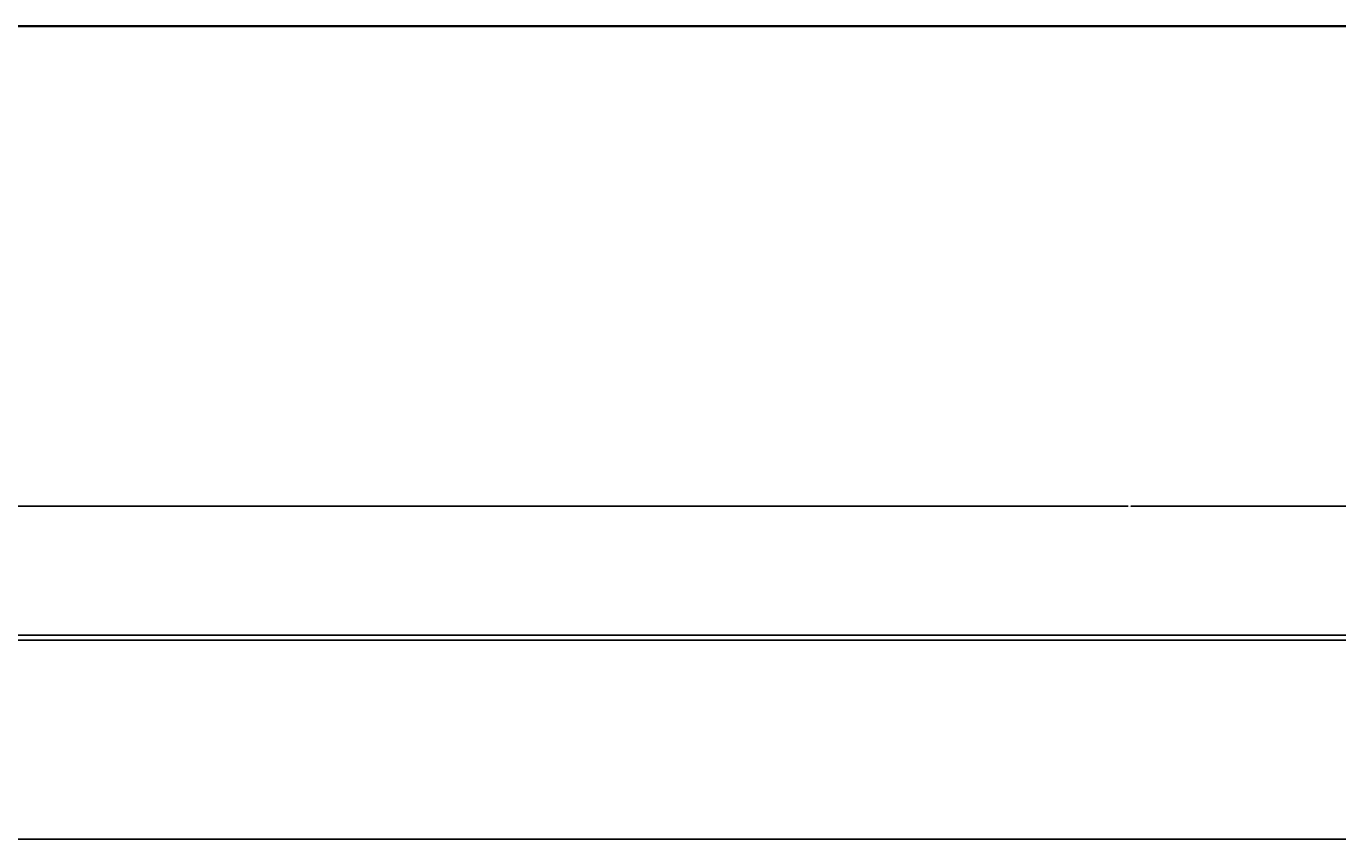
# Model space of a CAD drawing. Units: inches. Extents: x 1152 to 2588, y 1459 to 2618.
# Tile 13 of 17: x 1285 to 1548, y 2454 to 2618. Entities that reach past the tile are written whole.
import ezdxf

# ---------------------------------------------------------------- set-up
doc = ezdxf.new("R2010")
doc.units = ezdxf.units.IN
for name, color, linetype, lineweight in [('A-ANNO-DIMS', 2, 'Continuous', 18), ('A-ANNO-TTLB', 7, 'Continuous', 35), ('A-ELEV', 7, 'Continuous', 25)]:
    doc.layers.add(name, color=color, linetype=linetype, lineweight=lineweight)
doc.styles.get("Standard").update_dxf_attribs({"font": 'arial.ttf'})
doc.dimstyles.get("Standard").update_dxf_attribs({"dimtxt": 0.18, "dimasz": 0.18, "dimexe": 0.18, "dimexo": 0.0625, "dimgap": 0.09, "dimtad": 0, "dimtih": 1, "dimtoh": 1, "dimdec": 4, "dimzin": 0, "dimdsep": 46, "dimtxsty": 'Standard', "dimcen": 0.09, "dimadec": 0, "dimazin": 0, "dimtfac": 1, "dimtdec": 4, "dimtofl": 0, "dimtmove": 0, "dimatfit": 3, "dimfxl": 1, "dimtolj": 1, "dimtzin": 0, "dimarcsym": 0})

# ---------------------------------------------------------------- blocks, each defined once
blk = doc.blocks.new('*D88')
at = {"layer": 'A-ANNO-DIMS', "color": 0, "lineweight": -2, "transparency": 16777216}
for p, q in [((1252.42, 2495.45), (1252.42, 2521.47)), ((1252.6, 2521.29), (1506.13, 2521.29)), ((1760.24, 2521.29), (1506.71, 2521.29)), ((1760.42, 2495.45), (1760.42, 2521.47))]:
    blk.add_line(p, q, dxfattribs=at)
at = {"layer": 'A-ANNO-DIMS', "color": 0, "transparency": 16777216}
for points in [[(1252.6, 2521.32), (1252.6, 2521.26), (1252.42, 2521.29)], [(1760.24, 2521.32), (1760.24, 2521.26), (1760.42, 2521.29)]]:
    blk.add_solid(points, dxfattribs=at)
at = {"layer": 'Defpoints', "color": 0, "transparency": 16777216}
for p in [(1760.42, 2521.29), (1252.42, 2495.39), (1760.42, 2495.39)]:
    blk.add_point(p, dxfattribs=at)
at = {"layer": 'A-ANNO-DIMS', "color": 0, "transparency": 16777216, "insert": (1506.42, 2521.29), "char_height": 0.18, "attachment_point": 5}
blk.add_mtext('\\A1;508', dxfattribs=at)

msp = doc.modelspace()

# ---------------------------------------------------------------- linework, layer by layer
at = {"layer": 'A-ANNO-TTLB'}
msp.add_lwpolyline([(1152.3215, 2617.6685), (2587.6987, 2617.6685), (2587.6987, 1459.3148), (1152.3215, 1459.3148)], close=True, dxfattribs=at)
at = {"layer": 'A-ELEV'}
for p, q in [((1760.4165, 2495.3911), (1252.4165, 2495.3911)), ((1252.4165, 2494.3911), (1760.4165, 2494.3911)), ((1759.4165, 2454.3911), (1252.4165, 2454.3911))]:
    msp.add_line(p, q, dxfattribs=at)

# ---------------------------------------------------------------- dimensions: what is measured, and where the dimension line sits
at = {"layer": 'A-ANNO-DIMS'}
dim = msp.add_linear_dim(base=(1760.4165, 2521.2911), p1=(1252.4165, 2495.3911), p2=(1760.4165, 2495.3911), dimstyle='Standard', override={"dimdec": 0, "dimlfac": 1, "dimrnd": 0, "dimzin": 0, "dimdsep": 46, "dimlunit": 2}, dxfattribs=at)
dim.commit()
dim.dimension.update_dxf_attribs({"geometry": '*D88', "text_midpoint": (1506.4165, 2521.2911)})

doc.saveas('drawing.dxf')
